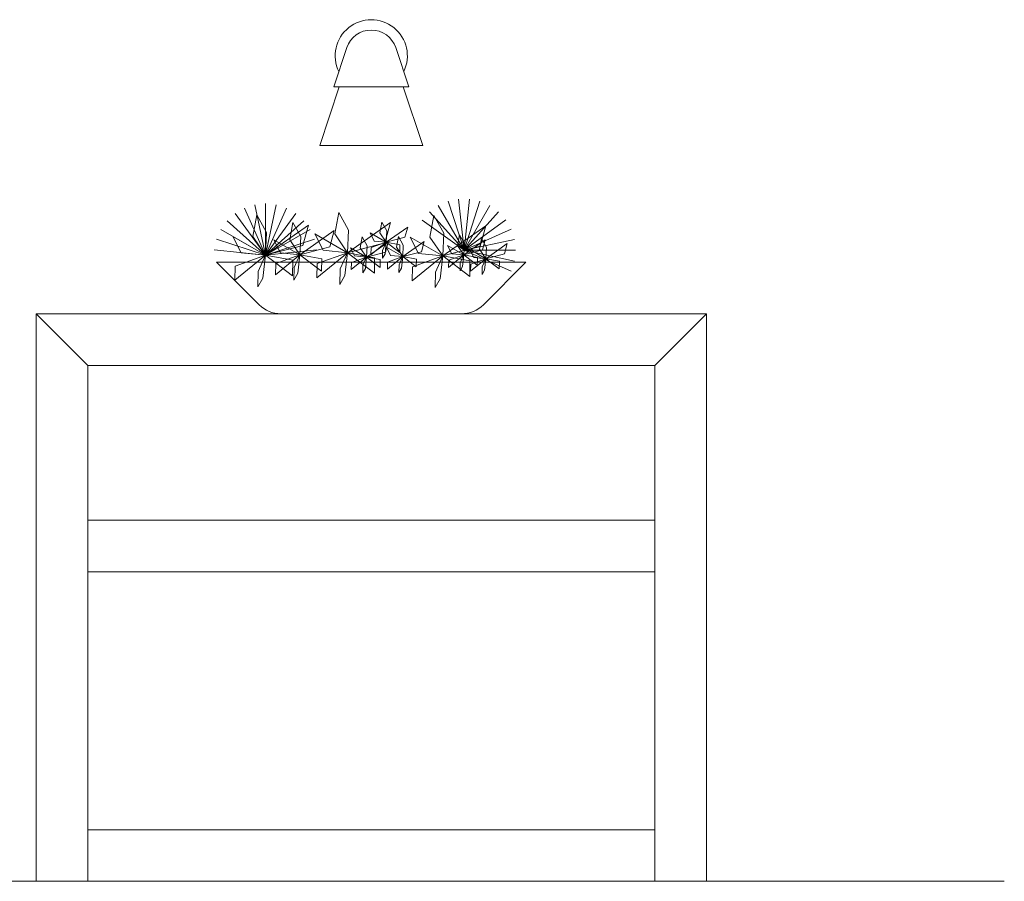
# Model space of a CAD drawing. Units: inches. Extents: x 1994 to 3075, y 3517 to 3950.
# Tile 29 of 58: x 1994.56485 to 1994.60244, y 3553.60329 to 3553.63617. Entities that reach past the tile are written whole.
import ezdxf

# ---------------------------------------------------------------- set-up
doc = ezdxf.new("R2010")
doc.units = ezdxf.units.IN
doc.layers.add('A-FURN-REFR', color=8, linetype='Continuous', lineweight=13)

msp = doc.modelspace()

# ---------------------------------------------------------------- linework, layer by layer
at = {"layer": 'A-FURN-REFR'}
for p, q in [((1994.576838600965, 3553.633608991265), (1994.577336051019, 3553.635101341428)), ((1994.57970098788, 3553.633608991265), (1994.579203537826, 3553.635101341428)), ((1994.576301290485, 3553.631374564225), (1994.577046099498, 3553.633608991265)), ((1994.57970098788, 3553.633608991264), (1994.576838600965, 3553.633608991265)), ((1994.580238298359, 3553.631374564225), (1994.579493489346, 3553.633608991265)), ((1994.580238298359, 3553.631374564225), (1994.576301290485, 3553.631374564225)), ((1994.581203004939, 3553.629240957197), (1994.581812462744, 3553.627369174909)), ((1994.581812462744, 3553.627369174909), (1994.581605488475, 3553.629326767666)), ((1994.582017017779, 3553.629327021937), (1994.581812462744, 3553.62736917491)), ((1994.581812462744, 3553.627369174909), (1994.582419607047, 3553.629241708899)), ((1994.57342983766, 3553.628979870546), (1994.574230500343, 3553.627181552716)), ((1994.574230500343, 3553.627181552716), (1994.573821225361, 3553.629107040119)), ((1994.574230500343, 3553.629150056654), (1994.574230500343, 3553.627181552716)), ((1994.574230500343, 3553.627181552716), (1994.574639775325, 3553.629107040119)), ((1994.575031163026, 3553.628979870546), (1994.574230500343, 3553.627181552716)), ((1994.581812462744, 3553.627369174909), (1994.580827157634, 3553.629073340861)), ((1994.582795661195, 3553.629074557141), (1994.581812462744, 3553.627369174909)), ((1994.572767616828, 3553.628498738949), (1994.574230500343, 3553.627181552716)), ((1994.574230500343, 3553.627181552716), (1994.57307344276, 3553.628774105855)), ((1994.573744505792, 3553.627900645149), (1994.573898556956, 3553.628721927778)), ((1994.573898556956, 3553.628721927778), (1994.574273160175, 3553.628048423386)), ((1994.574230500343, 3553.627181552716), (1994.575387557926, 3553.628774105855)), ((1994.575693383858, 3553.628498738949), (1994.574230500343, 3553.627181552716)), ((1994.576873399435, 3553.627996065702), (1994.5770274506, 3553.628817348331)), ((1994.5770274506, 3553.628817348331), (1994.577402053819, 3553.628143843938)), ((1994.581812462744, 3553.627369174909), (1994.580219194998, 3553.628525248281)), ((1994.58049437289, 3553.628831244294), (1994.581812462744, 3553.62736917491)), ((1994.580510833192, 3553.627872780074), (1994.580664884356, 3553.628694062704)), ((1994.580664884356, 3553.628694062704), (1994.581039487576, 3553.628020558311)), ((1994.581812462744, 3553.627369174909), (1994.583128744854, 3553.628832871995)), ((1994.583404300667, 3553.628527216263), (1994.581812462743, 3553.627369174909)), ((1994.574230500343, 3553.627181552716), (1994.572525725926, 3553.628165804685)), ((1994.57587125232, 3553.628330735697), (1994.574230500342, 3553.627181552715)), ((1994.574230500343, 3553.627181552716), (1994.57593527476, 3553.628165804685)), ((1994.575157892722, 3553.627775213666), (1994.575281133653, 3553.628432239769)), ((1994.575281133653, 3553.628432239769), (1994.575580816229, 3553.627893436255)), ((1994.576859289944, 3553.628119286104), (1994.575546688362, 3553.627199939718)), ((1994.575659484259, 3553.627559084138), (1994.57587125232, 3553.628330735697)), ((1994.576689875495, 3553.627501964856), (1994.576859289944, 3553.628119286104)), ((1994.579000145963, 3553.62842615625), (1994.577359393986, 3553.627276973268)), ((1994.577402053819, 3553.628143843938), (1994.577359393986, 3553.627276973268)), ((1994.578599841923, 3553.628035265095), (1994.578676867505, 3553.628445906411)), ((1994.578676867505, 3553.628445906411), (1994.578864169115, 3553.628109154214)), ((1994.578788377903, 3553.62765450469), (1994.579000145963, 3553.62842615625)), ((1994.579663215187, 3553.62825031037), (1994.578842839198, 3553.627675718879)), ((1994.578864169115, 3553.628109154214), (1994.578842839198, 3553.627675718879)), ((1994.579557331157, 3553.62786448459), (1994.579663215187, 3553.62825031037)), ((1994.58263757972, 3553.628302870623), (1994.580996827743, 3553.627153687641)), ((1994.581812462743, 3553.627369174909), (1994.583610285525, 3553.628170948567)), ((1994.582425811659, 3553.627531219063), (1994.58263757972, 3553.628302870623)), ((1994.572358341846, 3553.627789853886), (1994.574230500343, 3553.627181552716)), ((1994.574230500342, 3553.627181552715), (1994.572989026257, 3553.627897717092)), ((1994.572989026257, 3553.627897717092), (1994.57330591259, 3553.627273843752)), ((1994.574230500342, 3553.627181552715), (1994.573744505792, 3553.627900645149)), ((1994.574273160175, 3553.628048423386), (1994.574230500342, 3553.627181552715)), ((1994.57610265884, 3553.627789853886), (1994.574230500343, 3553.627181552716)), ((1994.575546688362, 3553.627199939718), (1994.574553509094, 3553.62777287122)), ((1994.574553509094, 3553.62777287122), (1994.57480701816, 3553.627273772548)), ((1994.575546688362, 3553.627199939718), (1994.575157892722, 3553.627775213666)), ((1994.575580816229, 3553.627893436255), (1994.575546688362, 3553.627199939718)), ((1994.577359393986, 3553.627276973268), (1994.576117919901, 3553.627993137644)), ((1994.576117919901, 3553.627993137644), (1994.576434806234, 3553.627369264305)), ((1994.577359393986, 3553.627276973268), (1994.576873399435, 3553.627996065702)), ((1994.577849605955, 3553.627468032783), (1994.577926631537, 3553.627878674098)), ((1994.577926631537, 3553.627878674098), (1994.578113933147, 3553.627541921902)), ((1994.578842839198, 3553.627675718879), (1994.578222102155, 3553.628033801067)), ((1994.578222102155, 3553.628033801067), (1994.578380545322, 3553.627721864398)), ((1994.578380545322, 3553.627721864398), (1994.578842839198, 3553.627675718879)), ((1994.578842839198, 3553.627675718879), (1994.578599841923, 3553.628035265095)), ((1994.578842839198, 3553.627675718879), (1994.579557331157, 3553.62786448459)), ((1994.579228412498, 3553.627488291979), (1994.57930543808, 3553.627898933294)), ((1994.57930543808, 3553.627898933294), (1994.57949273969, 3553.627562181097)), ((1994.580996827743, 3553.627153687641), (1994.579755353657, 3553.627869852017)), ((1994.579755353657, 3553.627869852017), (1994.58007223999, 3553.627245978677)), ((1994.580996827743, 3553.627153687641), (1994.580510833192, 3553.627872780074)), ((1994.581039487576, 3553.628020558311), (1994.580996827743, 3553.627153687641)), ((1994.581560814962, 3553.627552938169), (1994.581637840544, 3553.627963579483)), ((1994.581637840544, 3553.627963579483), (1994.581825142154, 3553.627626827287)), ((1994.582624188226, 3553.627767983443), (1994.581803812238, 3553.627193391952)), ((1994.583737696901, 3553.627779639515), (1994.581812462745, 3553.627369174909)), ((1994.582400168034, 3553.627408810954), (1994.582477193616, 3553.627819452269)), ((1994.582477193616, 3553.627819452269), (1994.582664495226, 3553.627482700072)), ((1994.582518304196, 3553.627382157664), (1994.582624188226, 3553.627767983443)), ((1994.574230500343, 3553.627181552716), (1994.572272780077, 3553.627387317408)), ((1994.574230500342, 3553.627181552715), (1994.575659484259, 3553.627559084138)), ((1994.574230500343, 3553.627181552716), (1994.576188220609, 3553.627387317408)), ((1994.575546688362, 3553.627199939718), (1994.576689875495, 3553.627501964856)), ((1994.576434806234, 3553.627369264305), (1994.577359393986, 3553.627276973268)), ((1994.577359393986, 3553.627276973268), (1994.578788377903, 3553.62765450469)), ((1994.57809260323, 3553.627108486566), (1994.577471866188, 3553.627466568754)), ((1994.577471866188, 3553.627466568754), (1994.577630309354, 3553.627154632085)), ((1994.57809260323, 3553.627108486566), (1994.577849605955, 3553.627468032783)), ((1994.578912979219, 3553.627683078057), (1994.57809260323, 3553.627108486566)), ((1994.578113933147, 3553.627541921902), (1994.57809260323, 3553.627108486566)), ((1994.578257931771, 3553.62719983195), (1994.578842839198, 3553.627675718879)), ((1994.578264553751, 3553.627470223645), (1994.578257931771, 3553.62719983195)), ((1994.578842839198, 3553.627675718879), (1994.578264553751, 3553.627470223645)), ((1994.578704053609, 3553.627368382612), (1994.578699453129, 3553.627071153961)), ((1994.578842839198, 3553.627675718879), (1994.578704053609, 3553.627368382612)), ((1994.578794672165, 3553.627240262041), (1994.578842839198, 3553.627675718879)), ((1994.578807095189, 3553.627297252277), (1994.578912979219, 3553.627683078057)), ((1994.578842839198, 3553.627675718879), (1994.579362850066, 3553.627579942366)), ((1994.579358249591, 3553.627282713637), (1994.578842839198, 3553.627675718879)), ((1994.579471409774, 3553.627128745762), (1994.578850672731, 3553.627486827951)), ((1994.578850672731, 3553.627486827951), (1994.579009115897, 3553.627174891281)), ((1994.579471409774, 3553.627128745762), (1994.579228412498, 3553.627488291979)), ((1994.579362850066, 3553.627579942366), (1994.579358249591, 3553.627282713637)), ((1994.580291785762, 3553.627703337253), (1994.579471409774, 3553.627128745762)), ((1994.57949273969, 3553.627562181097), (1994.579471409774, 3553.627128745762)), ((1994.580185901732, 3553.627317511473), (1994.580291785762, 3553.627703337253)), ((1994.580996827743, 3553.627153687641), (1994.582425811659, 3553.627531219063)), ((1994.581803812238, 3553.627193391952), (1994.581183075195, 3553.627551474141)), ((1994.581183075195, 3553.627551474141), (1994.581341518362, 3553.62723953747)), ((1994.581803812238, 3553.627193391952), (1994.581560814962, 3553.627552938169)), ((1994.581825142154, 3553.627626827287), (1994.581803812238, 3553.627193391952)), ((1994.581803812238, 3553.627193391952), (1994.582518304196, 3553.627382157664)), ((1994.581812462745, 3553.627369174909), (1994.583780966305, 3553.627370391189)), ((1994.581812462744, 3553.62736917491), (1994.583611274936, 3553.626569623506)), ((1994.583738202658, 3553.626961089707), (1994.581812462744, 3553.62736917491)), ((1994.582643165309, 3553.627049264738), (1994.582022428266, 3553.627407346925)), ((1994.582022428266, 3553.627407346925), (1994.582180871433, 3553.627095410256)), ((1994.582643165309, 3553.627049264738), (1994.582400168034, 3553.627408810954)), ((1994.583463541298, 3553.627623856228), (1994.582643165309, 3553.627049264738)), ((1994.582664495226, 3553.627482700072), (1994.582643165309, 3553.627049264738)), ((1994.583357657267, 3553.627238030449), (1994.583463541298, 3553.627623856228)), ((1994.573060685489, 3553.626229778858), (1994.574230500342, 3553.627181552715)), ((1994.574230500342, 3553.627181552715), (1994.573073929449, 3553.626770562247)), ((1994.57330591259, 3553.627273843752), (1994.574230500342, 3553.627181552715)), ((1994.574230500342, 3553.627181552715), (1994.573952929165, 3553.626566880183)), ((1994.574134166275, 3553.626310639039), (1994.574230500342, 3553.627181552715)), ((1994.574230500342, 3553.627181552715), (1994.575270522078, 3553.626989999689)), ((1994.575261321129, 3553.626395542231), (1994.574230500342, 3553.627181552715)), ((1994.57461083648, 3553.626438520633), (1994.575546688362, 3553.627199939718)), ((1994.575546688362, 3553.627199939718), (1994.574621431648, 3553.626871147343)), ((1994.57480701816, 3553.627273772548), (1994.575546688362, 3553.627199939718)), ((1994.575270522078, 3553.626989999689), (1994.575261321129, 3553.626395542231)), ((1994.575546688362, 3553.627199939718), (1994.57532463142, 3553.626708201692)), ((1994.575469621108, 3553.626503208778), (1994.575546688362, 3553.627199939718)), ((1994.575546688362, 3553.627199939718), (1994.576378705751, 3553.627046697297)), ((1994.576371344992, 3553.626571131332), (1994.575546688362, 3553.627199939718)), ((1994.576189579133, 3553.62632519941), (1994.577359393986, 3553.627276973268)), ((1994.577359393986, 3553.627276973268), (1994.576202823093, 3553.6268659828)), ((1994.576378705751, 3553.627046697297), (1994.576371344992, 3553.626571131332)), ((1994.577359393986, 3553.627276973268), (1994.577081822808, 3553.626662300735)), ((1994.577263059919, 3553.626406059591), (1994.577359393986, 3553.627276973268)), ((1994.577359393986, 3553.627276973268), (1994.578399415722, 3553.627085420242)), ((1994.578390214773, 3553.626490962784), (1994.577359393986, 3553.627276973268)), ((1994.577507695804, 3553.626632599637), (1994.57809260323, 3553.627108486566)), ((1994.57809260323, 3553.627108486566), (1994.577514317784, 3553.626902991332)), ((1994.577630309354, 3553.627154632085), (1994.57809260323, 3553.627108486566)), ((1994.57809260323, 3553.627108486566), (1994.577953817642, 3553.6268011503)), ((1994.578044436197, 3553.626673029728), (1994.57809260323, 3553.627108486566)), ((1994.57809260323, 3553.627108486566), (1994.578807095189, 3553.627297252277)), ((1994.57809260323, 3553.627108486566), (1994.578612614098, 3553.627012710053)), ((1994.578608013624, 3553.626715481325), (1994.57809260323, 3553.627108486566)), ((1994.578399415722, 3553.627085420242), (1994.578390214773, 3553.626490962784)), ((1994.578612614098, 3553.627012710053), (1994.578608013624, 3553.626715481325)), ((1994.578699453129, 3553.627071153961), (1994.578794672165, 3553.627240262041)), ((1994.578886502347, 3553.626652858833), (1994.579471409774, 3553.627128745762)), ((1994.579471409774, 3553.627128745762), (1994.578893124327, 3553.626923250528)), ((1994.579009115897, 3553.627174891281), (1994.579471409774, 3553.627128745762)), ((1994.579471409774, 3553.627128745762), (1994.579332624185, 3553.626821409495)), ((1994.57942324274, 3553.626693288924), (1994.579471409774, 3553.627128745762)), ((1994.579471409774, 3553.627128745762), (1994.580185901732, 3553.627317511473)), ((1994.579471409774, 3553.627128745762), (1994.579991420641, 3553.627032969249)), ((1994.579986820167, 3553.62673574052), (1994.579471409774, 3553.627128745762)), ((1994.579827012889, 3553.626201913783), (1994.580996827743, 3553.627153687641)), ((1994.580996827743, 3553.627153687641), (1994.579840256849, 3553.626742697173)), ((1994.579991420641, 3553.627032969249), (1994.579986820167, 3553.62673574052)), ((1994.58007223999, 3553.627245978677), (1994.580996827743, 3553.627153687641)), ((1994.580996827743, 3553.627153687641), (1994.580719256565, 3553.626539015108)), ((1994.580900493675, 3553.626282773964), (1994.580996827743, 3553.627153687641)), ((1994.580996827743, 3553.627153687641), (1994.582036849478, 3553.626962134615)), ((1994.582027648529, 3553.626367677158), (1994.580996827743, 3553.627153687641)), ((1994.581218904811, 3553.626717505024), (1994.581803812238, 3553.627193391952)), ((1994.581225526791, 3553.626987896718), (1994.581218904811, 3553.626717505024)), ((1994.581803812238, 3553.627193391952), (1994.581225526791, 3553.626987896718)), ((1994.581341518362, 3553.62723953747), (1994.581803812238, 3553.627193391952)), ((1994.581803812238, 3553.627193391952), (1994.581665026649, 3553.626886055686)), ((1994.581755645204, 3553.626757935114), (1994.581803812238, 3553.627193391952)), ((1994.581803812238, 3553.627193391952), (1994.582323823106, 3553.627097615439)), ((1994.582319222631, 3553.626800386711), (1994.581803812238, 3553.627193391952)), ((1994.582036849478, 3553.626962134615), (1994.582027648529, 3553.626367677158)), ((1994.582058257882, 3553.626573377808), (1994.582643165309, 3553.627049264738)), ((1994.582643165309, 3553.627049264738), (1994.582064879862, 3553.626843769503)), ((1994.582180871433, 3553.627095410256), (1994.582643165309, 3553.627049264738)), ((1994.582323823106, 3553.627097615439), (1994.582319222631, 3553.626800386711)), ((1994.582643165309, 3553.627049264738), (1994.58250437972, 3553.626741928471)), ((1994.582594998275, 3553.6266138079), (1994.582643165309, 3553.627049264738)), ((1994.582643165309, 3553.627049264738), (1994.583357657267, 3553.627238030449)), ((1994.582643165309, 3553.627049264738), (1994.583163176177, 3553.626953488225)), ((1994.583158575703, 3553.626656259496), (1994.582643165309, 3553.627049264738)), ((1994.584175306233, 3553.626916077879), (1994.572364282612, 3553.626916077879)), ((1994.573986849676, 3553.625293510814), (1994.572364282612, 3553.626916077879)), ((1994.573073929449, 3553.626770562247), (1994.573060685489, 3553.626229778858)), ((1994.574621431648, 3553.626871147343), (1994.57461083648, 3553.626438520633)), ((1994.57532463142, 3553.626708201692), (1994.575317270651, 3553.62623263585)), ((1994.576202823093, 3553.6268659828), (1994.576189579133, 3553.62632519941)), ((1994.577081822808, 3553.626662300735), (1994.577072621848, 3553.626067843433)), ((1994.577514317784, 3553.626902991332), (1994.577507695804, 3553.626632599637)), ((1994.577953817642, 3553.6268011503), (1994.577949217161, 3553.626503921649)), ((1994.577949217161, 3553.626503921649), (1994.578044436197, 3553.626673029728)), ((1994.578893124327, 3553.626923250528), (1994.578886502347, 3553.626652858833)), ((1994.579332624185, 3553.626821409495), (1994.579328023704, 3553.626524180844)), ((1994.579328023704, 3553.626524180844), (1994.57942324274, 3553.626693288924)), ((1994.579840256849, 3553.626742697173), (1994.579827012889, 3553.626201913783)), ((1994.581665026649, 3553.626886055686), (1994.581660426169, 3553.626588827035)), ((1994.581660426169, 3553.626588827035), (1994.581755645204, 3553.626757935114)), ((1994.582064879862, 3553.626843769503), (1994.582058257882, 3553.626573377808)), ((1994.58250437972, 3553.626741928471), (1994.58249977924, 3553.62644469982)), ((1994.58249977924, 3553.62644469982), (1994.582594998275, 3553.6266138079)), ((1994.582552739169, 3553.625293510814), (1994.584175306233, 3553.626916077879)), ((1994.583163176177, 3553.626953488225), (1994.583158575703, 3553.626656259496)), ((1994.573952929165, 3553.626566880183), (1994.573943728204, 3553.625972422881)), ((1994.573943728204, 3553.625972422881), (1994.574134166275, 3553.626310639039)), ((1994.575317270651, 3553.62623263585), (1994.575469621108, 3553.626503208778)), ((1994.577072621848, 3553.626067843433), (1994.577263059919, 3553.626406059591)), ((1994.580719256565, 3553.626539015108), (1994.580710055604, 3553.625944557806)), ((1994.580710055604, 3553.625944557806), (1994.580900493675, 3553.626282773964)), ((1994.565474518832, 3553.624947573942), (1994.565474518832, 3553.603294030634)), ((1994.565474518832, 3553.624947573942), (1994.591065070013, 3553.624947573942)), ((1994.567443022769, 3553.622979070004), (1994.565474518832, 3553.624947573942)), ((1994.581717573679, 3553.624947573942), (1994.574822015165, 3553.624947573941)), ((1994.589096566076, 3553.622979070004), (1994.591065070013, 3553.624947573942)), ((1994.591065070013, 3553.624947573942), (1994.591065070013, 3553.603294030634)), ((1994.567443022769, 3553.622979070004), (1994.567443022769, 3553.603294030634)), ((1994.567443022769, 3553.622979070004), (1994.589096566076, 3553.622979070004)), ((1994.589096566076, 3553.622979070004), (1994.589096566076, 3553.603294030634)), ((1994.567443022769, 3553.617073558193), (1994.589096566076, 3553.617073558193)), ((1994.567443022769, 3553.615105054257), (1994.589096566076, 3553.615105054257)), ((1994.567443022769, 3553.605262534571), (1994.589096566076, 3553.605262534571)), ((1994.602439621408, 3553.603294030634), (1994.442865031001, 3553.603294030634))]:
    msp.add_line(p, q, dxfattribs=at)
for centre, radius, start, end in [((1994.578269794422, 3553.634790093627), 0.0013779527559055, 334.0196402199972, 205.9803597800028), ((1994.578269794422, 3553.634790093627), 0.0009842519685039, 18.43494882292201, 161.565051177078), ((1994.574822015165, 3553.626128676304), 0.0011811023622047, 224.999999999298, 269.9999999996691), ((1994.581717573679, 3553.626128676304), 0.0011811023622047, 269.9999999996691, 314.9999999985961)]:
    msp.add_arc(centre, radius, start, end, dxfattribs=at)

doc.saveas('drawing.dxf')
